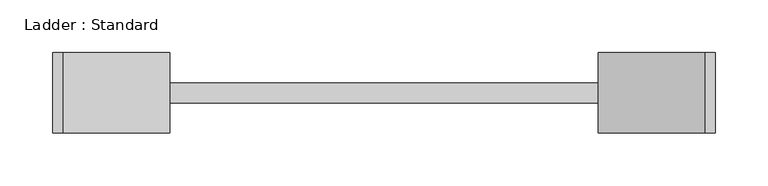
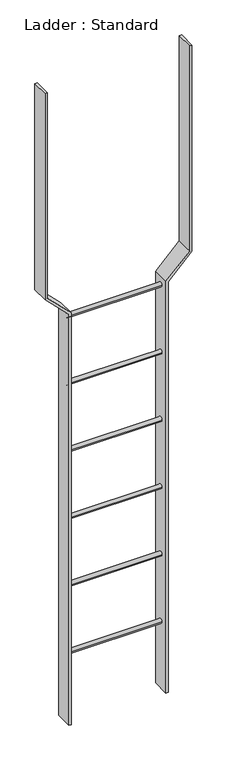
"""IFC4 building model written with IfcOpenShell, lengths in millimetres: proxy geometry, Ladder : Standard."""

from ifc_helpers import new_model, si_unit, point, frame, frame_2d, origin, place, context, project, spatial, polyline, circle_curve, trimmed, segment, composite_curve, outline, extrude, source, transform, mapped, element, save


def ladder_standard_86d3c5fc(model_context):
    return source(origin(), model_context, "Body", "SweptSolid", [
        extrude(outline(composite_curve([segment(trimmed(circle_curve(frame_2d((98.8219641, -1524.0)), 9.525), [point((89.2969641, -1524.0))], [point((108.3469641, -1524.0))], False, "CARTESIAN"), True, "CONTINUOUS"), segment(trimmed(circle_curve(frame_2d((98.8219641, -1524.0)), 9.525), [point((108.3469641, -1524.0))], [point((89.2969641, -1524.0))], False, "CARTESIAN"), True, "CONTINUOUS")], self_intersect=False)), frame((-203.2, 0.0, 0.0), z_axis=(1.0, 0.0, 0.0), x_axis=(0.0, 1.0, 0.0)), (0.0, 0.0, 1.0), 406.4),
        extrude(outline(composite_curve([segment(trimmed(circle_curve(frame_2d((98.8219641, -1219.2)), 9.525), [point((89.2969641, -1219.2))], [point((108.3469641, -1219.2))], False, "CARTESIAN"), True, "CONTINUOUS"), segment(trimmed(circle_curve(frame_2d((98.8219641, -1219.2)), 9.525), [point((108.3469641, -1219.2))], [point((89.2969641, -1219.2))], False, "CARTESIAN"), True, "CONTINUOUS")], self_intersect=False)), frame((-203.2, 0.0, 0.0), z_axis=(1.0, 0.0, 0.0), x_axis=(0.0, 1.0, 0.0)), (0.0, 0.0, 1.0), 406.4),
        extrude(outline(composite_curve([segment(trimmed(circle_curve(frame_2d((98.8219641, -914.4)), 9.525), [point((89.2969641, -914.4))], [point((108.3469641, -914.4))], False, "CARTESIAN"), True, "CONTINUOUS"), segment(trimmed(circle_curve(frame_2d((98.8219641, -914.4)), 9.525), [point((108.3469641, -914.4))], [point((89.2969641, -914.4))], False, "CARTESIAN"), True, "CONTINUOUS")], self_intersect=False)), frame((-203.2, 0.0, 0.0), z_axis=(1.0, 0.0, 0.0), x_axis=(0.0, 1.0, 0.0)), (0.0, 0.0, 1.0), 406.4),
        extrude(outline(composite_curve([segment(trimmed(circle_curve(frame_2d((98.8219641, -609.6)), 9.525), [point((89.2969641, -609.6))], [point((108.3469641, -609.6))], False, "CARTESIAN"), True, "CONTINUOUS"), segment(trimmed(circle_curve(frame_2d((98.8219641, -609.6)), 9.525), [point((108.3469641, -609.6))], [point((89.2969641, -609.6))], False, "CARTESIAN"), True, "CONTINUOUS")], self_intersect=False)), frame((-203.2, 0.0, 0.0), z_axis=(1.0, 0.0, 0.0), x_axis=(0.0, 1.0, 0.0)), (0.0, 0.0, 1.0), 406.4),
        extrude(outline(composite_curve([segment(trimmed(circle_curve(frame_2d((98.8219641, -304.8)), 9.525), [point((89.2969641, -304.8))], [point((108.3469641, -304.8))], False, "CARTESIAN"), True, "CONTINUOUS"), segment(trimmed(circle_curve(frame_2d((98.8219641, -304.8)), 9.525), [point((108.3469641, -304.8))], [point((89.2969641, -304.8))], False, "CARTESIAN"), True, "CONTINUOUS")], self_intersect=False)), frame((-203.2, 0.0, 0.0), z_axis=(1.0, 0.0, 0.0), x_axis=(0.0, 1.0, 0.0)), (0.0, 0.0, 1.0), 406.4),
        extrude(outline(composite_curve([segment(trimmed(circle_curve(frame_2d((98.8219641, 0.0)), 9.525), [point((89.2969641, 0.0))], [point((108.3469641, 0.0))], False, "CARTESIAN"), True, "CONTINUOUS"), segment(trimmed(circle_curve(frame_2d((98.8219641, 0.0)), 9.525), [point((108.3469641, 0.0))], [point((89.2969641, 0.0))], False, "CARTESIAN"), True, "CONTINUOUS")], self_intersect=False)), frame((-203.2, 0.0, 0.0), z_axis=(1.0, 0.0, 0.0), x_axis=(0.0, 1.0, 0.0)), (0.0, 0.0, 1.0), 406.4),
        extrude(outline(polyline([(1066.8, -314.325), (133.35, -314.325), (31.75, -212.725), (-1828.8, -212.725), (-1828.8, -203.2), (35.6953842, -203.2), (137.2953842, -304.8), (1066.8, -304.8), (1066.8, -314.325)])), frame((0.0, 60.7219641, 0.0), z_axis=(0.0, 1.0, 0.0), x_axis=(0.0, 0.0, 1.0)), (0.0, 0.0, 1.0), 76.2),
        extrude(outline(polyline([(1066.8, 304.8), (137.2953842, 304.8), (35.6953842, 203.2), (-1828.8, 203.2), (-1828.8, 212.725), (31.75, 212.725), (133.35, 314.325), (1066.8, 314.325), (1066.8, 304.8)])), frame((0.0, 60.7219641, 0.0), z_axis=(0.0, 1.0, 0.0), x_axis=(0.0, 0.0, 1.0)), (0.0, 0.0, 1.0), 76.2),
    ])


if __name__ == "__main__":
    model = new_model("IFC4")
    model_context = context("Model", 3, world=origin())
    ifc_project = project(units=[si_unit("LENGTHUNIT", "METRE", prefix="MILLI")], contexts=[model_context])
    site = spatial("IfcSite", under=ifc_project)
    building = spatial("IfcBuilding", under=site)
    placement = place(None, origin())
    ladder_standard_shape = ladder_standard_86d3c5fc(model_context)
    element("IfcBuildingElementProxy", 1, Name="Ladder : Standard", ObjectType="Ladder : Standard", at=placement, inside=building, context=model_context, shape_type="MappedRepresentation", body=[
        mapped(ladder_standard_shape, transform((0.0, 0.0, 0.0), x_axis=(1.0, 0.0, 0.0), y_axis=(0.0, 1.0, 0.0), z_axis=(0.0, 0.0, 1.0))),
    ])
    save(model, "model.ifc")

# Revit data of these elements
# Type "Ladder : Standard"
#   Rung Radius = 0' - 0 3/8"
#   Rung Length [instance default] = 1' - 4"
#   Side Rail Thickness = 0' - 3"
#   Side Rail Width = 0' - 0 3/8"
#   Half Guardrail Height = 1' - 9"
#   Height [instance default] = 15' - 2 1/2"
#   Guardrail Length = 1' - 8"
#   Guardrail Height = 3' - 6"
#   Distance [instance default] = 0' - 7"
#   Rung Space [instance default] = 1' - 0"
#   Number of Rungs [instance default] = 15
#   Default Elevation = 0
# Element 1 (IfcBuildingElementProxy, "Ladder : Standard")
#   Height = 6' - 0"
#   Distance = 0' - 1 25/64"
#   Number of Rungs = 6
